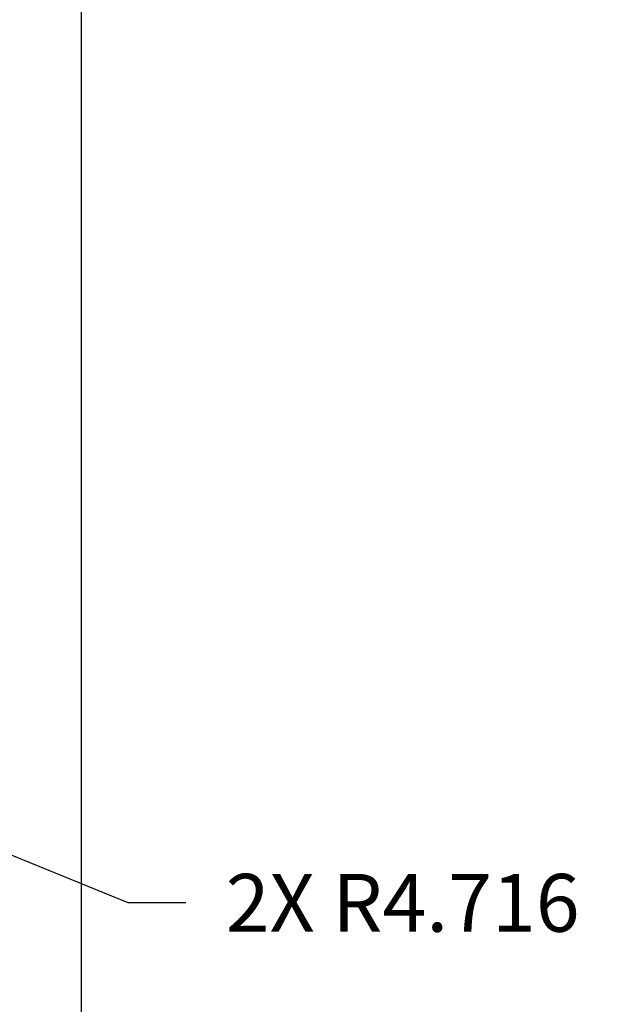
# Model space of a CAD drawing. Units: metres. Extents: x 4298.5 to 4325.2, y 2075 to 2095.8.
# Tile 25 of 35: x 4320.1 to 4321.9, y 2076.7 to 2079.7. Entities that reach past the tile are written whole.
import ezdxf

# ---------------------------------------------------------------- set-up
doc = ezdxf.new("R2010")
doc.units = ezdxf.units.M
doc.layers.add('A-ANNO-DIMS', color=2, linetype='Continuous', lineweight=18)
doc.styles.get("Standard").update_dxf_attribs({"font": 'arial.ttf'})
doc.dimstyles.get("Standard").update_dxf_attribs({"dimtxt": 0.18, "dimasz": 0.18, "dimexe": 0.18, "dimexo": 0.0625, "dimgap": 0.09, "dimtad": 0, "dimtih": 1, "dimtoh": 1, "dimdec": 4, "dimzin": 0, "dimdsep": 46, "dimtxsty": 'Standard', "dimcen": 0.09, "dimadec": 0, "dimazin": 0, "dimtfac": 1, "dimtdec": 4, "dimtofl": 0, "dimtmove": 0, "dimatfit": 3, "dimfxl": 1, "dimtolj": 1, "dimtzin": 0, "dimarcsym": 0})

# ---------------------------------------------------------------- blocks, each defined once
blk = doc.blocks.new('*D47')
at = {"layer": 'A-ANNO-DIMS', "color": 0, "lineweight": -2, "transparency": 16777216}
for p, q in [((4300.4306, 2084.4956), (4300.4306, 2074.9896)), ((4322.8106, 2084.4956), (4322.8106, 2074.9896)), ((4300.6106, 2075.1696), (4311.2252, 2075.1696)), ((4322.6306, 2075.1696), (4312.016, 2075.1696))]:
    blk.add_line(p, q, dxfattribs=at)
at = {"layer": 'A-ANNO-DIMS', "color": 0, "transparency": 16777216}
for points in [[(4300.6106, 2075.1996), (4300.6106, 2075.1396), (4300.4306, 2075.1696)], [(4322.6306, 2075.1996), (4322.6306, 2075.1396), (4322.8106, 2075.1696)]]:
    blk.add_solid(points, dxfattribs=at)
at = {"layer": 'Defpoints', "color": 0, "transparency": 16777216}
for p in [(4300.4306, 2084.5581), (4322.8106, 2084.5581), (4322.8106, 2075.1696)]:
    blk.add_point(p, dxfattribs=at)
at = {"layer": 'A-ANNO-DIMS', "color": 0, "transparency": 16777216, "insert": (4311.6206, 2075.1696), "char_height": 0.18, "attachment_point": 5}
blk.add_mtext('\\A1;22.38', dxfattribs=at)
blk = doc.blocks.new('*D48')
at = {"layer": 'A-ANNO-DIMS', "color": 0, "lineweight": -2, "transparency": 16777216}
for p, q in [((4310.1831, 2094.4781), (4324.7671, 2094.4781)), ((4324.5871, 2094.2981), (4324.5871, 2085.585)), ((4324.5871, 2076.5081), (4324.5871, 2085.2212)), ((4316.8731, 2076.3281), (4324.7671, 2076.3281))]:
    blk.add_line(p, q, dxfattribs=at)
at = {"layer": 'A-ANNO-DIMS', "color": 0, "transparency": 16777216}
for points in [[(4324.5571, 2094.2981), (4324.6171, 2094.2981), (4324.5871, 2094.4781)], [(4324.5571, 2076.5081), (4324.6171, 2076.5081), (4324.5871, 2076.3281)]]:
    blk.add_solid(points, dxfattribs=at)
at = {"layer": 'Defpoints', "color": 0, "transparency": 16777216}
for p in [(4310.1206, 2094.4781), (4316.8106, 2076.3281), (4324.5871, 2076.3281)]:
    blk.add_point(p, dxfattribs=at)
at = {"layer": 'A-ANNO-DIMS', "color": 0, "transparency": 16777216, "insert": (4324.5871, 2085.4031), "char_height": 0.18, "attachment_point": 5}
blk.add_mtext('\\A1;18.15', dxfattribs=at)
blk = doc.blocks.new('*D55')
at = {"layer": 'A-ANNO-DIMS', "color": 0, "lineweight": -2, "transparency": 16777216}
for p, q in [((4320.3167, 2084.4996), (4320.3167, 2074.9896)), ((4322.8106, 2084.4956), (4322.8106, 2074.9896)), ((4320.4967, 2075.1696), (4321.1688, 2075.1696)), ((4322.6306, 2075.1696), (4321.9585, 2075.1696))]:
    blk.add_line(p, q, dxfattribs=at)
at = {"layer": 'A-ANNO-DIMS', "color": 0, "transparency": 16777216}
for points in [[(4320.4967, 2075.1996), (4320.4967, 2075.1396), (4320.3167, 2075.1696)], [(4322.6306, 2075.1996), (4322.6306, 2075.1396), (4322.8106, 2075.1696)]]:
    blk.add_solid(points, dxfattribs=at)
at = {"layer": 'Defpoints', "color": 0, "transparency": 16777216}
for p in [(4320.3167, 2084.5621), (4322.8106, 2084.5581), (4322.8106, 2075.1696)]:
    blk.add_point(p, dxfattribs=at)
at = {"layer": 'A-ANNO-DIMS', "color": 0, "transparency": 16777216, "insert": (4321.5636, 2075.1696), "char_height": 0.18, "attachment_point": 5}
blk.add_mtext('\\A1;2.494', dxfattribs=at)
blk = doc.blocks.new('*D79')
at = {"layer": 'A-ANNO-DIMS', "color": 0, "lineweight": -2, "transparency": 16777216}
for p, q in [((4313.4743, 2079.7393), (4313.4743, 2079.9193)), ((4313.3843, 2079.8293), (4313.5643, 2079.8293)), ((4320.4622, 2076.981), (4318.0084, 2077.9812)), ((4320.6422, 2076.981), (4320.4622, 2076.981))]:
    blk.add_line(p, q, dxfattribs=at)
at = {"layer": 'A-ANNO-DIMS', "color": 0, "transparency": 16777216}
blk.add_solid([(4318.0197, 2078.009), (4317.9971, 2077.9534), (4317.8417, 2078.0491)], dxfattribs=at)
at = {"layer": 'Defpoints', "color": 0, "transparency": 16777216}
for p in [(4313.4743, 2079.8293), (4317.8417, 2078.0491)]:
    blk.add_point(p, dxfattribs=at)
at = {"layer": 'A-ANNO-DIMS', "color": 0, "transparency": 16777216, "insert": (4321.3169, 2076.981), "char_height": 0.18, "attachment_point": 5}
blk.add_mtext('\\A1;2X R4.716', dxfattribs=at)

msp = doc.modelspace()

# ---------------------------------------------------------------- dimensions: what is measured, and where the dimension line sits
at = {"layer": 'A-ANNO-DIMS'}
dim = msp.add_linear_dim(base=(4324.5871, 2076.3281), p1=(4310.1206, 2094.4781), p2=(4316.8106, 2076.3281), angle=90, dimstyle='Standard', override={"dimdec": 2, "dimlfac": 1, "dimrnd": 0, "dimzin": 0, "dimdsep": 46, "dimlunit": 2}, dxfattribs=at)
dim.commit()
dim.dimension.update_dxf_attribs({"geometry": '*D48', "text_midpoint": (4324.5871, 2085.4031)})
for p1, override, picture, middle in [((4300.4306, 2084.5581), {"dimdec": 2, "dimlfac": 1, "dimrnd": 0, "dimzin": 0, "dimdsep": 46, "dimlunit": 2}, '*D47', (4311.6206, 2075.1696)), ((4320.3167, 2084.5621), {"dimdec": 3, "dimlfac": 1, "dimrnd": 0, "dimzin": 0, "dimdsep": 46, "dimlunit": 2}, '*D55', (4321.5636, 2075.1696))]:
    dim = msp.add_linear_dim(base=(4322.8106, 2075.1696), p1=p1, p2=(4322.8106, 2084.5581), dimstyle='Standard', override=override, dxfattribs=at)
    dim.commit()
    dim.dimension.update_dxf_attribs({"geometry": picture, "text_midpoint": middle})
dim = msp.add_radius_dim(center=(4313.4743, 2079.8293), mpoint=(4317.8417, 2078.0491), text='2X <>', dimstyle='Standard', override={"dimdec": 3, "dimlfac": 1, "dimrnd": 0, "dimzin": 0, "dimdsep": 46, "dimlunit": 2}, dxfattribs=at)
dim.commit()
dim.dimension.update_dxf_attribs({"geometry": '*D79', "text_midpoint": (4321.3169, 2076.981), "dimtype": 164})

doc.saveas('drawing.dxf')
